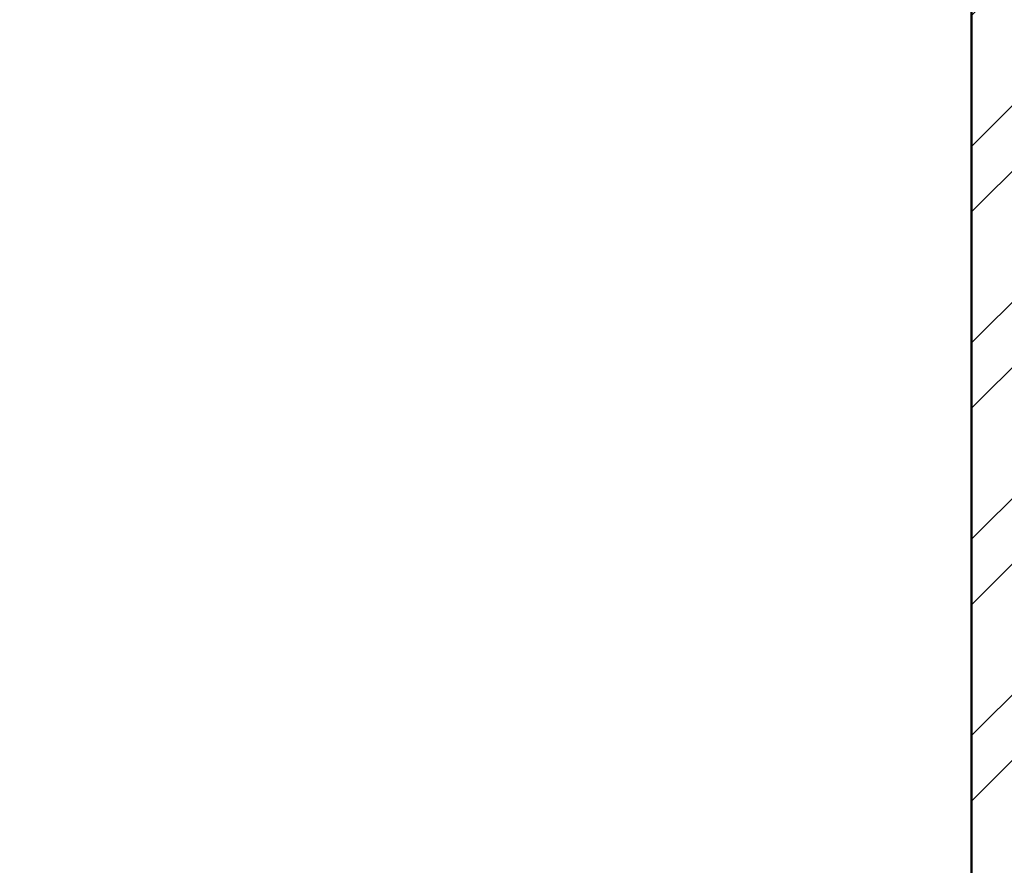
# Model space of a CAD drawing. Units: inches. Extents: x 1901 to 2863, y 888 to 2433.
# Tile 25 of 91: x 2540 to 2607, y 1289 to 1347. Entities that reach past the tile are written whole.
import ezdxf

# ---------------------------------------------------------------- set-up
doc = ezdxf.new("R2010")
doc.units = ezdxf.units.IN
doc.layers.add('A-WALL', color=7, linetype='Continuous', lineweight=50)
doc.layers.add('A-WALL-PATT', color=8, linetype='Continuous', lineweight=13)

msp = doc.modelspace()

# ---------------------------------------------------------------- hatches: boundary and pattern name
at = {"layer": 'A-WALL-PATT'}
h = msp.add_hatch(dxfattribs=at)
h.set_pattern_fill('ANSI32', color=256)
h.paths.add_polyline_path([(2443.926, 2139.888), (2439.426, 2139.888), (2439.426, 2069.348), (2441.676, 2069.348), (2443.926, 2069.348), (2443.926, 2078.634), (2521.926, 2078.634), (2521.926, 2075.067), (2524.176, 2075.067), (2526.426, 2075.067), (2526.426, 2078.634), (2571.755, 2078.634), (2571.755, 2080.884), (2571.755, 2083.134), (2443.926, 2083.134)])
h.paths.add_polyline_path([(2526.426, 2054.634), (2524.176, 2054.634), (2521.926, 2054.634), (2521.926, 2030.634), (2443.926, 2030.634), (2443.926, 2045.348), (2439.426, 2045.348), (2439.426, 1983.867), (2443.926, 1983.867), (2443.926, 2026.134), (2521.926, 2026.134), (2526.426, 2026.134)])
h.paths.add_polyline_path([(2443.926, 1923.867), (2439.426, 1923.867), (2439.426, 1872.634), (2443.926, 1872.634)])
h.paths.add_polyline_path([(2636.233, 1766.134), (2609.926, 1766.134), (2609.926, 1779.785), (2605.426, 1779.785), (2605.426, 1766.134), (2486.614, 1766.134), (2486.614, 1770.671), (2482.114, 1770.671), (2482.114, 1766.134), (2482.114, 1761.634), (2636.233, 1761.634), (2636.233, 1763.884)])
h.paths.add_polyline_path([(2519.536, 1663.384), (2519.536, 1665.634), (2494.926, 1665.634), (2481.831, 1665.634), (2481.831, 1663.384), (2481.831, 1661.134), (2490.426, 1661.134), (2490.426, 1640.157), (2494.926, 1640.157), (2494.926, 1661.134), (2519.536, 1661.134)])
h.paths.add_polyline_path([(2443.926, 1712.134), (2443.926, 1716.634), (2414.464, 1716.634), (2414.464, 1712.134), (2439.426, 1712.134), (2439.426, 1545.507), (2443.926, 1545.507), (2443.926, 1661.134), (2448.475, 1661.134), (2448.475, 1665.634), (2443.926, 1665.634)])
h.paths.add_polyline_path([(2343.426, 1712.134), (2365.525, 1712.134), (2365.525, 1714.384), (2365.525, 1716.634), (2333.871, 1716.634), (2333.871, 1714.384), (2333.871, 1712.134), (2338.926, 1712.134), (2338.926, 1575.634), (2338.926, 1545.507), (2343.426, 1545.507), (2343.426, 1547.507), (2343.426, 1580.134)])
h.paths.add_polyline_path([(2752.926, 1665.634), (2579.536, 1665.634), (2579.536, 1661.134), (2615.926, 1661.134), (2615.926, 1529.134), (2598.931, 1529.134), (2598.931, 1524.634), (2623.127, 1524.634), (2623.127, 1526.884), (2623.127, 1529.134), (2620.426, 1529.134), (2620.426, 1661.134), (2748.426, 1661.134), (2748.426, 1633.499), (2752.926, 1633.499)])
h.paths.add_polyline_path([(2752.926, 1419.929), (2748.426, 1419.929), (2748.426, 1400.134), (2659.426, 1400.134), (2659.426, 1444.333), (2657.176, 1444.333), (2654.926, 1444.333), (2654.926, 1400.134), (2643.649, 1400.134), (2643.649, 1395.634), (2748.426, 1395.634), (2748.426, 1364.035), (2752.926, 1364.035)])
h.paths.add_polyline_path([(2752.926, 1492.878), (2748.426, 1492.878), (2748.426, 1476.634), (2667.426, 1476.634), (2667.426, 1479.71), (2665.176, 1479.71), (2662.926, 1479.71), (2662.926, 1476.634), (2654.926, 1476.634), (2654.926, 1469.536), (2659.426, 1469.536), (2659.426, 1472.134), (2748.426, 1472.134), (2748.426, 1455.929), (2752.926, 1455.929)])
h.paths.add_polyline_path([(2752.926, 1304.035), (2748.426, 1304.035), (2748.426, 1263.634), (2738.66, 1263.634), (2738.66, 1259.134), (2752.926, 1259.134)])
h.paths.add_polyline_path([(2685.926, 1259.134), (2695.49, 1259.134), (2695.49, 1261.384), (2695.49, 1263.634), (2677.837, 1263.634), (2677.837, 1261.384), (2677.837, 1259.134), (2681.426, 1259.134), (2681.426, 1203.634), (2653.277, 1203.634), (2653.277, 1199.134), (2685.926, 1199.134), (2685.926, 1203.634)])
h.paths.add_polyline_path([(2609.426, 1395.634), (2611.848, 1395.634), (2611.848, 1400.134), (2598.888, 1400.134), (2598.888, 1397.884), (2598.888, 1395.634), (2604.926, 1395.634), (2604.926, 1268.134), (2554.726, 1268.134), (2554.726, 1265.884), (2554.726, 1263.634), (2604.926, 1263.634), (2604.926, 1203.634), (2571.306, 1203.634), (2571.306, 1199.134), (2604.926, 1199.134), (2629.277, 1199.134), (2629.277, 1201.384), (2629.277, 1203.634), (2609.426, 1203.634), (2609.426, 1258.634), (2609.426, 1259.134), (2654.804, 1259.134), (2654.804, 1263.634), (2609.426, 1263.634)])
h.paths.add_polyline_path([(2443.926, 1304.035), (2439.426, 1304.035), (2439.426, 1259.134), (2443.926, 1259.134), (2456.16, 1259.134), (2456.16, 1261.384), (2456.16, 1263.634), (2443.926, 1263.634)])
h.paths.add_polyline_path([(2525.426, 1263.634), (2531.778, 1263.634), (2531.778, 1268.134), (2520.926, 1268.134), (2520.926, 1263.634), (2511.409, 1263.634), (2511.409, 1259.134), (2520.926, 1259.134), (2520.926, 1199.134), (2547.306, 1199.134), (2547.306, 1201.384), (2547.306, 1203.634), (2525.426, 1203.634)])
h.paths.add_polyline_path([(2443.926, 1434.842), (2439.426, 1434.842), (2439.426, 1364.035), (2441.676, 1364.035), (2443.926, 1364.035)])
h.paths.add_polyline_path([(2567.134, 1400.134), (2443.926, 1400.134), (2443.926, 1395.634), (2567.134, 1395.634)])
h.paths.add_polyline_path([(2443.926, 1545.507), (2439.426, 1545.507), (2439.426, 1494.842), (2443.926, 1494.842)])
h.paths.add_polyline_path([(2494.926, 1553.349), (2492.676, 1553.349), (2490.426, 1553.349), (2490.426, 1524.634), (2494.926, 1524.634), (2525.936, 1524.634), (2525.936, 1526.884), (2525.936, 1529.134), (2494.926, 1529.134)])
h.paths.add_polyline_path([(2752.926, 1573.499), (2748.426, 1573.499), (2748.426, 1529.134), (2657.759, 1529.134), (2657.759, 1524.634), (2662.926, 1524.634), (2662.926, 1498.631), (2667.426, 1498.631), (2667.426, 1524.634), (2748.426, 1524.634), (2748.426, 1516.878), (2752.926, 1516.878)])
h.paths.add_polyline_path([(2038.602, 2237.418), (2080.174, 2237.418), (2080.174, 2256.075), (2038.602, 2256.075)], flags=9)
h.paths.add_polyline_path([(2292.009, 1062.394), (2539.932, 1062.394), (2539.932, 1099.487), (2292.009, 1099.487)], flags=9)
h.paths.add_polyline_path([(2424.91, 1832.253), (2448.513, 1832.253), (2448.513, 1846.678), (2424.91, 1846.678)], flags=9)
h.paths.add_polyline_path([(2359.076, 1832.253), (2382.678, 1832.253), (2382.678, 1846.678), (2359.076, 1846.678)], flags=9)
h.paths.add_polyline_path([(2352.899, 1684.802), (2367.543, 1684.802), (2367.543, 1697.167), (2352.899, 1697.167)], flags=9)
h.paths.add_polyline_path([(2079.288, 1755.826), (2169.024, 1755.826), (2169.024, 1774.372), (2079.288, 1774.372)], flags=9)
h.paths.add_polyline_path([(2404.09, 1373.857), (2404.09, 1463.593), (2385.544, 1463.593), (2385.544, 1373.857)], flags=9)
h.paths.add_polyline_path([(2268.091, 2236.371), (2309.636, 2236.371), (2309.636, 2255.028), (2268.091, 2255.028)], flags=9)
h.paths.add_polyline_path([(2575.96, 1700.951), (2665.696, 1700.951), (2665.696, 1719.498), (2575.96, 1719.498)], flags=9)
h.paths.add_polyline_path([(2302.962, 1878.474), (2329.524, 1878.474), (2329.524, 1888.777), (2302.962, 1888.777)], flags=9)
h.paths.add_polyline_path([(2097.415, 2240.576), (2126.573, 2240.576), (2126.573, 2259.233), (2097.415, 2259.233)], flags=9)
h.paths.add_polyline_path([(2208.725, 2246.124), (2237.882, 2246.124), (2237.882, 2264.781), (2208.725, 2264.781)], flags=9)
h.paths.add_polyline_path([(2038.147, 1925.958), (2076.987, 1925.958), (2076.987, 1944.615), (2038.147, 1944.615)], flags=9)
h.paths.add_polyline_path([(2239.144, 1926.672), (2288.465, 1926.672), (2288.465, 1945.329), (2239.144, 1945.329)], flags=9)
h.paths.add_polyline_path([(2175.429, 2007.33), (2212.356, 2007.33), (2212.356, 2025.987), (2175.429, 2025.987)], flags=9)
h.paths.add_polyline_path([(2225.034, 2091.794), (2263.875, 2091.794), (2263.875, 2110.451), (2225.034, 2110.451)], flags=9)
h.paths.add_polyline_path([(2035.398, 2098.478), (2074.238, 2098.478), (2074.238, 2117.135), (2035.398, 2117.135)], flags=9)
h.paths.add_polyline_path([(2050.102, 2029.209), (2083.26, 2029.209), (2083.26, 2047.866), (2050.102, 2047.866)], flags=9)
h.paths.add_polyline_path([(2069.677, 1956.719), (2098.835, 1956.719), (2098.835, 1975.376), (2069.677, 1975.376)], flags=9)
h.paths.add_polyline_path([(2328.62, 1753.336), (2361.663, 1753.336), (2361.663, 1771.993), (2328.62, 1771.993)], flags=9)
h.paths.add_polyline_path([(2395.162, 2060.888), (2395.162, 2140.654), (2378.676, 2140.654), (2378.676, 2060.888)], flags=9)
h.paths.add_polyline_path([(2463.728, 2059.02), (2492.886, 2059.02), (2492.886, 2077.677), (2463.728, 2077.677)], flags=9)
h.paths.add_polyline_path([(2458.027, 2181.536), (2496.868, 2181.536), (2496.868, 2200.194), (2458.027, 2200.194)], flags=9)
h.paths.add_polyline_path([(2456.855, 2228.831), (2498.401, 2228.831), (2498.401, 2247.488), (2456.855, 2247.488)], flags=9)
h.paths.add_polyline_path([(2527.577, 2243.074), (2556.735, 2243.074), (2556.735, 2261.731), (2527.577, 2261.731)], flags=9)
h.paths.add_polyline_path([(2694.461, 2232.767), (2736.033, 2232.767), (2736.033, 2251.425), (2694.461, 2251.425)], flags=9)
h.paths.add_polyline_path([(2637.821, 2249.225), (2666.979, 2249.225), (2666.979, 2267.882), (2637.821, 2267.882)], flags=9)
h.paths.add_polyline_path([(2623.687, 2183.541), (2662.528, 2183.541), (2662.528, 2202.199), (2623.687, 2202.199)], flags=9)
h.paths.add_polyline_path([(2691.965, 2021.5), (2725.124, 2021.5), (2725.124, 2040.157), (2691.965, 2040.157)], flags=9)
h.paths.add_polyline_path([(2621.043, 1975.912), (2662.335, 1975.912), (2662.335, 1994.569), (2621.043, 1994.569)], flags=9)
h.paths.add_polyline_path([(2479.032, 1927.62), (2519.844, 1927.62), (2519.844, 1946.277), (2479.032, 1946.277)], flags=9)
h.paths.add_polyline_path([(2670.941, 1849.076), (2716.005, 1849.076), (2716.005, 1867.734), (2670.941, 1867.734)], flags=9)
h.paths.add_polyline_path([(2523.613, 1782.956), (2550.175, 1782.956), (2550.175, 1793.26), (2523.613, 1793.26)], flags=9)
h.paths.add_polyline_path([(2450.841, 1207.331), (2492.386, 1207.331), (2492.386, 1225.989), (2450.841, 1225.989)], flags=9)
h.paths.add_polyline_path([(2527.751, 1203.841), (2556.908, 1203.841), (2556.908, 1222.499), (2527.751, 1222.499)], flags=9)
h.paths.add_polyline_path([(2639.111, 1207.2), (2668.268, 1207.2), (2668.268, 1225.857), (2639.111, 1225.857)], flags=9)
h.paths.add_polyline_path([(2692.594, 1218.965), (2734.167, 1218.965), (2734.167, 1237.623), (2692.594, 1237.623)], flags=9)
h.paths.add_polyline_path([(2669.266, 1366.329), (2708.106, 1366.329), (2708.106, 1384.987), (2669.266, 1384.987)], flags=25)
h.paths.add_polyline_path([(2463.313, 1358.031), (2502.153, 1358.031), (2502.153, 1376.688), (2463.313, 1376.688)], flags=9)
h.paths.add_polyline_path([(2494.725, 1449.963), (2531.652, 1449.963), (2531.652, 1468.62), (2494.725, 1468.62)], flags=9)
h.paths.add_polyline_path([(2675.565, 1422.157), (2708.724, 1422.157), (2708.724, 1440.815), (2675.565, 1440.815)], flags=25)
h.paths.add_polyline_path([(2685.634, 1493.891), (2714.792, 1493.891), (2714.792, 1512.548), (2685.634, 1512.548)], flags=9)
h.paths.add_polyline_path([(2686.805, 1529.913), (2725.645, 1529.913), (2725.645, 1548.57), (2686.805, 1548.57)], flags=25)
h.paths.add_polyline_path([(2503.651, 1537.991), (2552.972, 1537.991), (2552.972, 1556.648), (2503.651, 1556.648)], flags=9)
h.paths.add_polyline_path([(2291.713, 1643.504), (2318.275, 1643.504), (2318.275, 1653.807), (2291.713, 1653.807)], flags=9)
h.paths.add_polyline_path([(2450.626, 1610.52), (2477.189, 1610.52), (2477.189, 1620.824), (2450.626, 1620.824)], flags=9)
h.paths.add_polyline_path([(2359.985, 1551.814), (2422.253, 1551.814), (2422.253, 1562.117), (2359.985, 1562.117)], flags=9)
h.paths.add_polyline_path([(2280.106, 1249.006), (2321.651, 1249.006), (2321.651, 1267.663), (2280.106, 1267.663)], flags=9)
h.paths.add_polyline_path([(2164.057, 1274.232), (2193.215, 1274.232), (2193.215, 1292.889), (2164.057, 1292.889)], flags=9)
h.paths.add_polyline_path([(2118.21, 1277.694), (2151.252, 1277.694), (2151.252, 1296.351), (2118.21, 1296.351)], flags=9)
h.paths.add_polyline_path([(2031.946, 1268.529), (2073.519, 1268.529), (2073.519, 1287.187), (2031.946, 1287.187)], flags=9)
h.paths.add_polyline_path([(2050.199, 1409.079), (2089.04, 1409.079), (2089.04, 1427.736), (2050.199, 1427.736)], flags=9)
h.paths.add_polyline_path([(2243.743, 1421.032), (2282.584, 1421.032), (2282.584, 1439.689), (2243.743, 1439.689)], flags=9)
h.paths.add_polyline_path([(2190.746, 1509.769), (2231.558, 1509.769), (2231.558, 1528.426), (2190.746, 1528.426)], flags=9)
h.paths.add_polyline_path([(2058.392, 1475.415), (2091.55, 1475.415), (2091.55, 1494.073), (2058.392, 1494.073)], flags=9)
h.paths.add_polyline_path([(2062.447, 1553.09), (2091.605, 1553.09), (2091.605, 1571.747), (2062.447, 1571.747)], flags=9)
h.paths.add_polyline_path([(2219.524, 1590.365), (2266.147, 1590.365), (2266.147, 1609.022), (2219.524, 1609.022)], flags=9)
h.paths.add_polyline_path([(2041.072, 1584.188), (2079.912, 1584.188), (2079.912, 1602.845), (2041.072, 1602.845)], flags=9)

# ---------------------------------------------------------------- linework, layer by layer
at = {"layer": 'A-WALL'}
msp.add_line((2604.926, 1395.634), (2604.926, 1268.134), dxfattribs=at)

doc.saveas('drawing.dxf')
